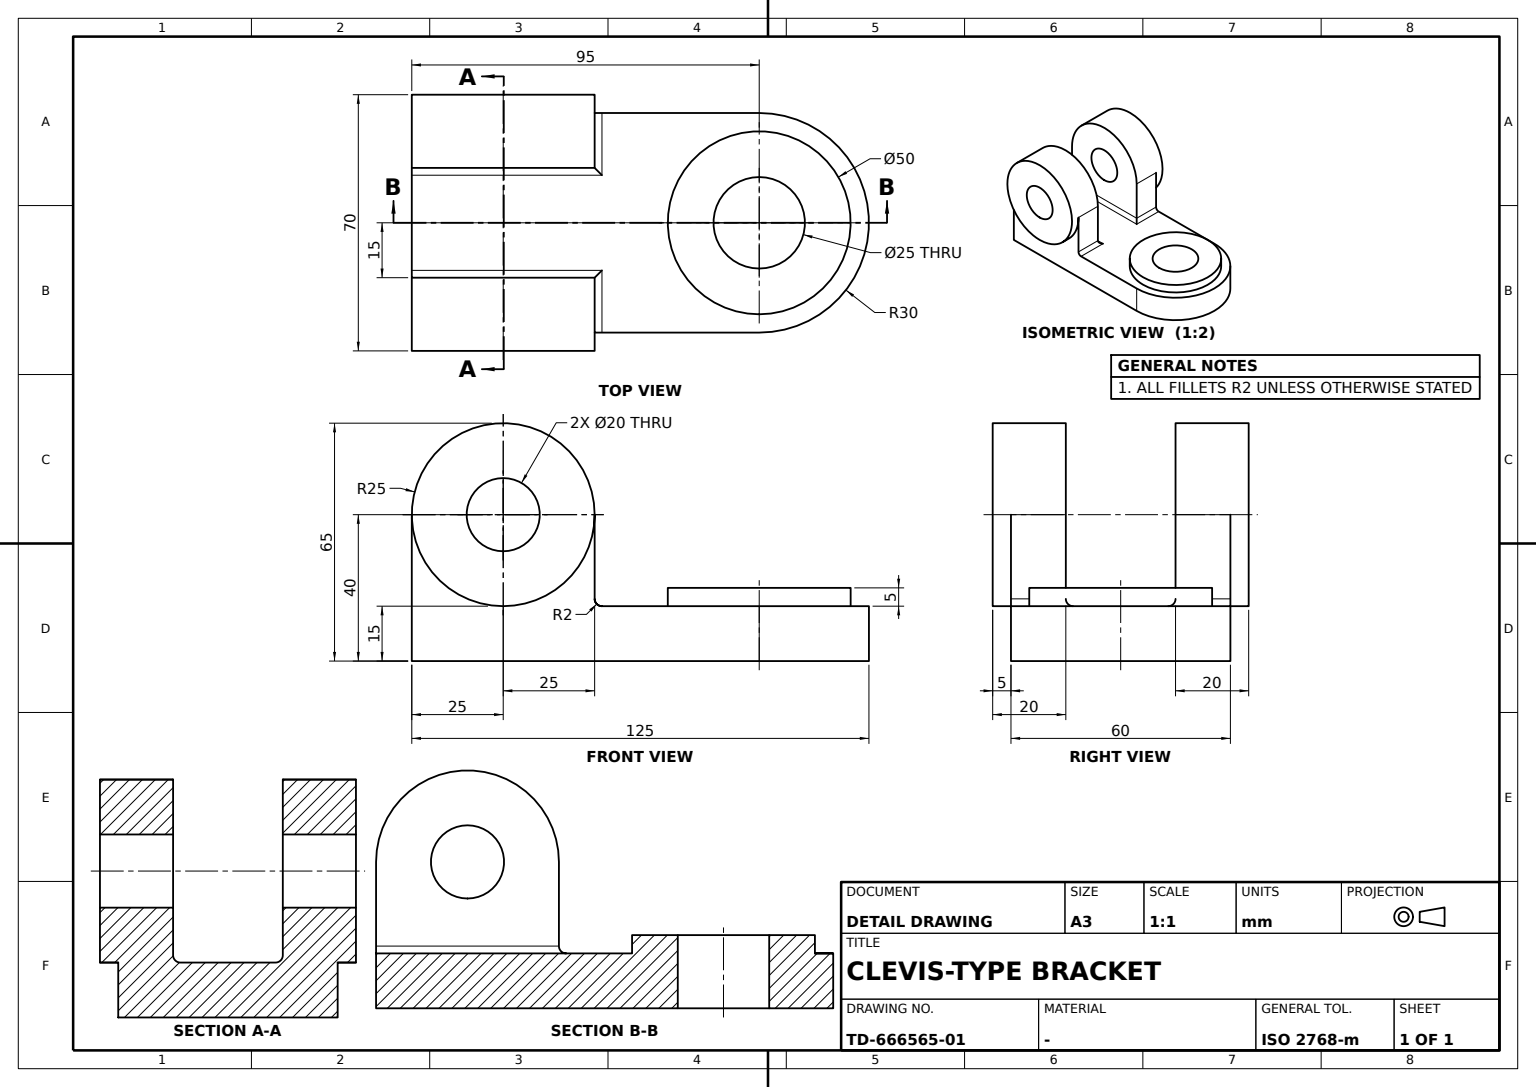
CATIA V5 part; units mm, degrees
sketch "Sketch1" plane through (0, 0, 0) normal (0, 0, 1) x (1, 0, 0)
  arc A0 (30, 0) -> (-30, 0) centre (0, 0) ccw
  point P0 (-30, 0)
  line L0 (-30, 0) -> (-30, -95)
  line L1 (-30, -95) -> (30, -95)
  line L2 (30, -95) -> (30, 0)
  point P1 (30, 0)
  dimension "radius A0" = 30
  dimension "length L0" = 95
  constraint coincidence P0 x-axis
  constraint coincidence P1 x-axis
  constraint tangency L0 A0
  constraint horizontal L1 x-axis
  constraint vertical L2 y-axis
extrude "Pad1" add sketch "Sketch1" along normal blind 15
sketch "Sketch2" plane through (0, 0, 15) normal (0, 0, 1) x (1, 0, 0)
  arc A0 (30, 0) -> (-30, 0) centre (0, 0) ccw construction
  circle A1 centre (0, 0) radius 25
  dimension "radius A1" = 25
  constraint concentricity A1 A0
extrude "Pad2" add sketch "Sketch2" along normal blind 5
sketch "Sketch3" plane through (0, 0, 20) normal (0, 0, 1) x (1, 0, 0)
  point P0 (0, 0)
hole "Hole1" at (0, 0, 20) direction (0, 0, -1) diameter 25 depth 20
sketch "Sketch4" plane through (30, 0, 0) normal (1, 0, 0) x (0, 1, 0)
  arc A0 (-45, 40) -> (-95, 40) centre (-70, 40) ccw
  point P0 (-70, 40)
  line L0 (-95, 40) -> (-95, 15)
  point P1 (-95, 15)
  line L1 (-95, 15) -> (-45, 15)
  line L2 (-45, 15) -> (-45, 40)
  line L3 (-95, 15) -> (0, 15) construction
  point P2 (-95, 15)
  dimension "radius A0" = 25
  dimension "distance P0 L1" = 25
  constraint tangency L0 A0
  constraint tangency L2 A0
  constraint horizontal L1 x-axis
  constraint vertical L2 y-axis
  constraint coincidence L1 L3
  constraint coincidence P2 P1
extrude "Pad3" add sketch "Sketch4" against normal blind 15
sketch "Sketch5" plane through (30, 0, 0) normal (1, 0, 0) x (0, 1, 0)
  arc A0 (-45, 40) -> (-95, 40) centre (-70, 40) ccw construction
  circle A1 centre (-70, 40) radius 25
  constraint concentricity A1 A0
  constraint coincidence A0 A1
extrude "Pad4" add sketch "Sketch5" along normal blind 5
sketch "Sketch6" plane through (35, -70, 40) normal (1, 0, 0) x (0, 1, 0)
  point P0 (0, 0)
hole "Hole2" at (35, -70, 40) direction (-1, 0, 0) diameter 20 depth 20
mirror "Mirror1" about plane through (0, 0, 0) normal (1, 0, 0) of "Pad3"
sketch "Sketch7" plane through (-30, 0, 0) normal (-1, 0, 0) x (0, -1, 0)
  circle A0 centre (70, 40) radius 25
  arc A1 (95, 40) -> (45, 40) centre (70, 40) ccw construction
  arc A2 (95, 40) -> (45, 40) centre (70, 40) ccw construction
  constraint concentricity A0 A1
  constraint coincidence A2 A0
extrude "Pad5" add sketch "Sketch7" along normal blind 5
sketch "Sketch8" plane through (-35, -70, 40) normal (-1, 0, 0) x (0, 1, 0)
  point P0 (0, 0)
hole "Hole3" at (-35, -70, 40) direction (1, 0, 0) diameter 20 depth 20
fillet "Fillet1" radius 2 1 edges at (22.5, -45, 15)
fillet "Fillet2" radius 2 1 edges at (-22.5, -45, 15)
fillet "Fillet3" radius 2 1 edges at (-15, -70, 15)
fillet "Fillet4" radius 2 1 edges at (15, -70, 15)
